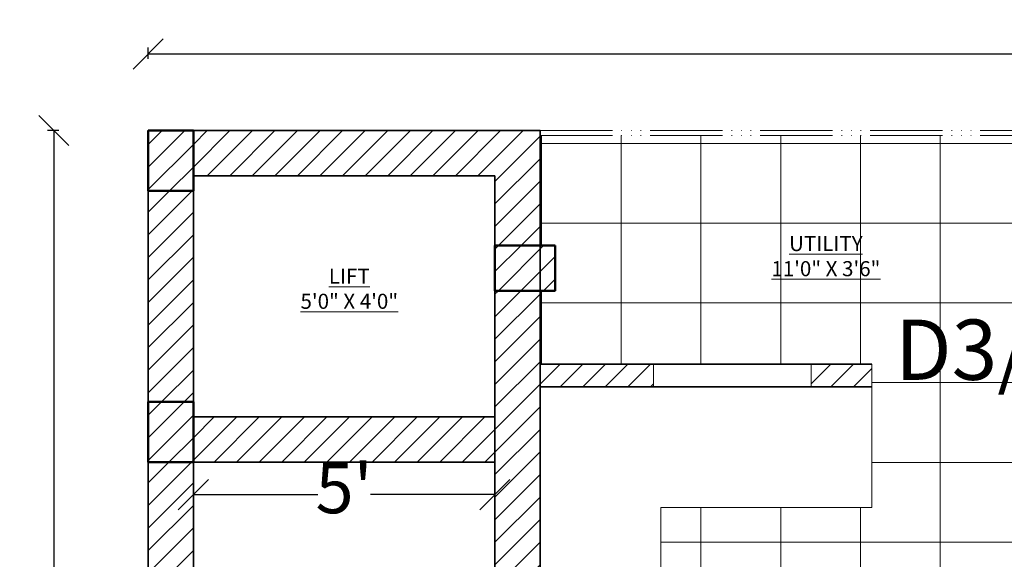
# Model space of a CAD drawing. Units: inches. Extents: x 2036 to 2670, y 319 to 920.
# Tile 4 of 15: x 2055 to 2251, y 790 to 898. Entities that reach past the tile are written whole.
import ezdxf

# ---------------------------------------------------------------- set-up
doc = ezdxf.new("R2010")
doc.units = ezdxf.units.IN
doc.linetypes.add('ACAD_ISO06W100', pattern=[36, 24, -3, 0, -3, 0, -3, 0, -3])
for name, color, linetype, lineweight in [('A-ANNO-DIMS', 2, 'Continuous', 18), ('A-ANNO-TEXT', 7, 'Continuous', 18), ('A-AREA-IDEN', 7, 'Continuous', 18), ('A-CASE', 7, 'Continuous', 18), ('A-COLS', 7, 'Continuous', 50), ('A-FLOR-EDGE', 5, 'ACAD_ISO06W100', 13), ('A-FLOR-PATT', 8, 'Continuous', 9), ('A-GLAZ', 4, 'Continuous', 18), ('A-WALL', 7, 'Continuous', 35)]:
    doc.layers.add(name, color=color, linetype=linetype, lineweight=lineweight)
doc.layers.add('A-COLS-PATT', color=240, linetype='Continuous', lineweight=13, true_color=0xed1f24)
doc.layers.add('A-WALL-PATT', color=52, linetype='Continuous', lineweight=13, true_color=0xc8c92d)
doc.styles.get("Standard").update_dxf_attribs({"font": 'arial.ttf'})
doc.dimstyles.new('ISO-25', dxfattribs={"dimtxt": 10, "dimasz": 6, "dimexe": 1.25, "dimexo": 0.625, "dimtad": 0, "dimdec": 1, "dimlunit": 3, "dimtxsty": 'Standard', "dimblk": 'OBLIQUE', "dimcen": 2.5, "dimclrd": 94, "dimclre": 94, "dimclrt": 1, "dimadec": 0, "dimazin": 0, "dimtfac": 1, "dimtdec": 1, "dimtmove": 0, "dimatfit": 3, "dimfxl": 1, "dimfxlon": 1, "dimarcsym": 0})

# ---------------------------------------------------------------- blocks, each defined once
blk = doc.blocks.new('_Oblique')
at = {"color": 0, "linetype": 'ByBlock', "lineweight": -2}
blk.add_line((-0.5, -0.5), (0.5, 0.5), dxfattribs=at)
blk = doc.blocks.new('*D10')
at = {"layer": 'A-ANNO-DIMS', "color": 0, "lineweight": -2, "transparency": 16777216}
for p, q in [((2080.74, 889.93), (2080.74, 892.18)), ((2612.74, 889.93), (2612.74, 892.18)), ((2080.74, 890.93), (2328.73, 890.93)), ((2612.74, 890.93), (2364.74, 890.93))]:
    blk.add_line(p, q, dxfattribs=at)
at = {"layer": 'Defpoints', "color": 0, "transparency": 16777216}
for p in [(2612.74, 890.93), (2080.74, 875.68), (2612.74, 875.68)]:
    blk.add_point(p, dxfattribs=at)
at = {"layer": 'A-ANNO-DIMS', "color": 0, "lineweight": -2, "transparency": 16777216, "xscale": 6, "yscale": 6, "zscale": 6, "rotation": 180}
blk.add_blockref('_Oblique', (2080.74, 890.93), dxfattribs=at)
at = {"layer": 'A-ANNO-DIMS', "color": 0, "lineweight": -2, "transparency": 16777216, "xscale": 6, "yscale": 6, "zscale": 6}
blk.add_blockref('_Oblique', (2612.74, 890.93), dxfattribs=at)
at = {"layer": 'A-ANNO-DIMS', "color": 0, "transparency": 16777216, "insert": (2346.74, 890.93), "char_height": 10, "attachment_point": 5}
blk.add_mtext('44\'-4"', dxfattribs=at)
blk = doc.blocks.new('*D13')
at = {"layer": 'A-ANNO-DIMS', "color": 0, "lineweight": -2, "transparency": 16777216}
for p, q in [((2062.98, 875.68), (2060.73, 875.68)), ((2061.98, 875.68), (2061.98, 687.98)), ((2061.98, 464.68), (2061.98, 652.39)), ((2062.98, 464.68), (2060.73, 464.68))]:
    blk.add_line(p, q, dxfattribs=at)
at = {"layer": 'Defpoints', "color": 0, "transparency": 16777216}
for p in [(2080.74, 875.68), (2061.98, 464.68), (2080.74, 464.68)]:
    blk.add_point(p, dxfattribs=at)
at = {"layer": 'A-ANNO-DIMS', "color": 0, "lineweight": -2, "transparency": 16777216, "xscale": 6, "yscale": 6, "zscale": 6}
for p, rotation in [((2061.98, 875.68), 90), ((2061.98, 464.68), 270)]:
    blk.add_blockref('_Oblique', p, dxfattribs=dict(at, rotation=rotation))
at = {"layer": 'A-ANNO-DIMS', "color": 0, "transparency": 16777216, "insert": (2061.98, 670.18), "char_height": 10, "attachment_point": 5, "rotation": 90}
blk.add_mtext('34\'-3"', dxfattribs=at)
blk = doc.blocks.new('*D14')
at = {"layer": 'A-ANNO-DIMS', "color": 0, "lineweight": -2, "transparency": 16777216}
for p, q in [((2089.74, 804.21), (2089.74, 801.96)), ((2149.74, 804.21), (2149.74, 801.96)), ((2089.74, 803.21), (2114.51, 803.21)), ((2149.74, 803.21), (2124.96, 803.21))]:
    blk.add_line(p, q, dxfattribs=at)
at = {"layer": 'Defpoints', "color": 0, "transparency": 16777216}
for p in [(2089.74, 809.68), (2149.74, 809.68), (2149.74, 803.21)]:
    blk.add_point(p, dxfattribs=at)
at = {"layer": 'A-ANNO-DIMS', "color": 0, "lineweight": -2, "transparency": 16777216, "xscale": 6, "yscale": 6, "zscale": 6, "rotation": 180}
blk.add_blockref('_Oblique', (2089.74, 803.21), dxfattribs=at)
at = {"layer": 'A-ANNO-DIMS', "color": 0, "lineweight": -2, "transparency": 16777216, "xscale": 6, "yscale": 6, "zscale": 6}
blk.add_blockref('_Oblique', (2149.74, 803.21), dxfattribs=at)
at = {"layer": 'A-ANNO-DIMS', "color": 0, "transparency": 16777216, "insert": (2119.74, 803.21), "char_height": 10, "attachment_point": 5}
blk.add_mtext("5'", dxfattribs=at)
blk = doc.blocks.new('COL-9x12')
blk.add_lwpolyline([(9, 0), (0, 0), (0, 12), (9, 12)], close=True)
blk = doc.blocks.new('*D58')
at = {"layer": 'A-ANNO-DIMS', "color": 94, "lineweight": -2, "transparency": 16777216}
for p, q in [((2224.74, 436.33), (2224.74, 434.08)), ((2224.74, 435.33), (2270.11, 435.33)), ((2270.11, 436.33), (2270.11, 434.08)), ((2270.11, 435.33), (2276.11, 435.33))]:
    blk.add_line(p, q, dxfattribs=at)
at = {"layer": 'Defpoints', "color": 0, "transparency": 16777216}
for p in [(2224.74, 824.68), (2270.11, 824.68), (2270.11, 435.33)]:
    blk.add_point(p, dxfattribs=at)
at = {"layer": 'A-ANNO-DIMS', "color": 94, "lineweight": -2, "transparency": 16777216, "xscale": 6, "yscale": 6, "zscale": 6, "rotation": 180}
blk.add_blockref('_Oblique', (2224.74, 435.33), dxfattribs=at)
at = {"layer": 'A-ANNO-DIMS', "color": 94, "lineweight": -2, "transparency": 16777216, "xscale": 6, "yscale": 6, "zscale": 6}
blk.add_blockref('_Oblique', (2270.11, 435.33), dxfattribs=at)
at = {"layer": 'A-ANNO-DIMS', "color": 1, "transparency": 16777216, "insert": (2301.68, 435.33), "char_height": 10, "attachment_point": 5}
blk.add_mtext('3\'-9 1/2"', dxfattribs=at)

msp = doc.modelspace()

# ---------------------------------------------------------------- hatches: boundary and pattern name
at = {"layer": 'A-COLS-PATT'}
h = msp.add_hatch(dxfattribs=at)
h.set_pattern_fill('ANSI31', color=256)
h.paths.add_polyline_path([(2089.74, 875.68), (2080.74, 875.68), (2080.74, 863.68), (2089.74, 863.68)])
h.paths.add_polyline_path([(2089.74, 821.68), (2080.74, 821.68), (2080.74, 809.68), (2089.74, 809.68)])
h.paths.add_polyline_path([(2089.74, 624.2), (2080.74, 624.2), (2080.74, 612.2), (2089.74, 612.2)])
h.paths.add_polyline_path([(2158.74, 506.68), (2149.74, 506.68), (2149.74, 494.68), (2158.74, 494.68)])
h.paths.add_polyline_path([(2158.74, 617.33), (2149.74, 617.33), (2149.74, 605.33), (2158.74, 605.33)])
h.paths.add_polyline_path([(2158.74, 736.18), (2149.74, 736.18), (2149.74, 724.18), (2158.74, 724.18)])
h.paths.add_polyline_path([(2158.74, 852.81), (2149.74, 852.81), (2149.74, 843.81), (2158.74, 843.81)])
h.paths.add_polyline_path([(2161.74, 852.81), (2158.74, 852.81), (2158.74, 843.81), (2161.74, 843.81)])
h.paths.add_polyline_path([(2295.21, 857.66), (2290.74, 857.66), (2290.74, 848.68), (2295.21, 848.68)])
h.paths.add_polyline_path([(2290.74, 857.66), (2283.21, 857.66), (2283.21, 848.66), (2290.74, 848.66)])
h.paths.add_polyline_path([(2443.62, 857.68), (2431.62, 857.68), (2431.62, 848.68), (2443.62, 848.68)])
h.paths.add_polyline_path([(2561.81, 857.68), (2549.81, 857.68), (2549.81, 848.68), (2561.81, 848.68)])
h.paths.add_polyline_path([(2295.24, 737.65), (2290.74, 737.65), (2290.74, 728.68), (2295.24, 728.68)])
h.paths.add_polyline_path([(2309.27, 612.12), (2297.27, 612.12), (2297.27, 603.12), (2309.27, 603.12)])
h.paths.add_polyline_path([(2282.24, 503.68), (2270.24, 503.68), (2270.24, 494.68), (2282.24, 494.68)])
h.paths.add_polyline_path([(2431.74, 746.09), (2427.24, 746.09), (2427.24, 737.09), (2431.74, 737.09)])
h.paths.add_polyline_path([(2439.24, 746.09), (2431.74, 746.09), (2431.74, 737.09), (2439.24, 737.09)])
h.paths.add_polyline_path([(2596.59, 736.59), (2584.59, 736.59), (2584.59, 727.59), (2596.59, 727.59)])
h.paths.add_polyline_path([(2586.39, 623.71), (2574.39, 623.71), (2574.39, 619.18), (2586.39, 619.18)])
h.paths.add_polyline_path([(2586.39, 619.18), (2574.39, 619.18), (2574.39, 614.71), (2586.39, 614.71)])
h.paths.add_polyline_path([(2438.74, 623.68), (2431.24, 623.68), (2431.24, 619.18), (2438.74, 619.18)])
h.paths.add_polyline_path([(2438.74, 619.18), (2431.24, 619.18), (2431.24, 614.68), (2438.74, 614.68)])
h.paths.add_polyline_path([(2431.24, 623.68), (2426.74, 623.68), (2426.74, 614.68), (2431.24, 614.68), (2431.24, 619.18)])
h.paths.add_polyline_path([(2527.24, 503.68), (2515.24, 503.68), (2515.24, 494.68), (2527.24, 494.68)])
h.paths.add_polyline_path([(2590.31, 503.68), (2578.31, 503.68), (2578.31, 494.68), (2590.31, 494.68)])
at = {"layer": 'A-FLOR-PATT'}
h = msp.add_hatch(dxfattribs=at)
h.set_pattern_fill('ANSI31', color=256, scale=5, angle=135)
h.paths.add_polyline_path([(2290.74, 659.68), (2158.74, 659.68), (2158.74, 582.53), (2158.74, 545.51), (2158.74, 503.68), (2426.74, 503.68), (2426.74, 614.68), (2426.74, 623.68), (2426.74, 628.18), (2431.24, 628.18), (2431.24, 623.68), (2438.74, 623.68), (2438.74, 619.18), (2574.39, 619.18), (2574.39, 623.71), (2586.39, 623.71), (2586.39, 619.18), (2603.74, 619.18), (2603.74, 824.68), (2431.74, 824.68), (2431.74, 746.09), (2439.24, 746.09), (2439.24, 737.09), (2431.74, 737.09), (2431.74, 659.68), (2427.24, 659.68), (2427.24, 739.48), (2383.24, 739.48), (2383.24, 804.68), (2339.24, 804.68), (2339.24, 749.08), (2295.24, 749.08), (2295.24, 737.65), (2295.27, 737.65), (2295.27, 728.65), (2295.21, 728.65, -0.586418), (2272.74, 728.68), (2272.74, 824.68), (2270.11, 824.68), (2270.11, 829.18), (2290.74, 829.18), (2290.74, 848.66), (2283.21, 848.66), (2283.21, 857.66), (2289.74, 857.66), (2289.74, 874.68), (2158.74, 874.68), (2158.74, 852.81), (2161.74, 852.81), (2161.74, 843.81), (2158.74, 843.81), (2158.74, 829.18), (2224.74, 829.18), (2224.74, 800.68), (2182.74, 800.68), (2182.74, 733.41), (2158.74, 733.41), (2158.74, 728.68), (2235.24, 728.68), (2235.24, 714.81), (2230.74, 714.81), (2230.74, 724.18), (2158.74, 724.18), (2158.74, 664.18), (2230.74, 664.18), (2230.74, 678.81), (2235.24, 678.81), (2235.24, 664.18), (2290.74, 664.18)])
h.paths.add_polyline_path([(2309.27, 612.12), (2309.27, 603.12), (2297.27, 603.12), (2297.27, 612.12)], flags=16)
h.paths.add_polyline_path([(2280.12, 639.11), (2280.26, 638.18, -0.414214), (2279.26, 637.18), (2278.76, 637.18), (2279.26, 633.18), (2277.76, 633.18), (2277.26, 637.18), (2269.76, 637.18), (2262.26, 637.18), (2261.76, 633.18), (2260.26, 633.18), (2260.76, 637.18), (2260.26, 637.18, -0.414214), (2259.26, 638.18), (2259.41, 639.11, -0.541164), (2257.76, 641.18), (2260.76, 652.18), (2261.45, 652.18), (2261.53, 652.68), (2262.76, 652.68), (2262.25, 655.24, 0.001913), (2261.76, 655.18), (2259.76, 658.18, -0.15), (2279.76, 658.18), (2277.76, 655.18, 0.001913), (2277.27, 655.24), (2276.76, 652.68), (2278, 652.68), (2278.07, 652.18), (2278.76, 652.18), (2281.76, 641.18, -0.541163)], flags=16)
h.paths.add_polyline_path([(2245.98, 639.11), (2246.13, 638.18, -0.414214), (2245.13, 637.18), (2244.63, 637.18), (2245.13, 633.18), (2243.63, 633.18), (2243.13, 637.18), (2235.63, 637.18), (2228.13, 637.18), (2227.63, 633.18), (2226.13, 633.18), (2226.63, 637.18), (2226.13, 637.18, -0.414214), (2225.13, 638.18), (2225.27, 639.11, -0.541164), (2223.63, 641.18), (2226.63, 652.18), (2227.32, 652.18), (2227.39, 652.68), (2228.63, 652.68), (2228.12, 655.24, 0.001913), (2227.63, 655.18), (2225.63, 658.18, -0.15), (2245.63, 658.18), (2243.63, 655.18, 0.001913), (2243.14, 655.24), (2242.63, 652.68), (2243.86, 652.68), (2243.94, 652.18), (2244.63, 652.18), (2247.63, 641.18, -0.541163)], flags=16)
h.paths.add_polyline_path([(2351.59, 515.15, -0.151948), (2279.59, 515.15), (2279.59, 537.68), (2273.59, 537.68), (2273.59, 511.68, 0.190476), (2357.59, 511.68), (2357.59, 537.68), (2351.59, 537.68)])
h.paths.add_polyline_path([(2327.59, 536.13), (2327.59, 517.07), (2303.59, 517.07), (2303.59, 536.13)], flags=16)
h.paths.add_polyline_path([(2213.4, 639.11), (2213.55, 638.18, -0.414214), (2212.55, 637.18), (2212.05, 637.18), (2212.55, 633.18), (2211.05, 633.18), (2210.55, 637.18), (2203.05, 637.18), (2195.55, 637.18), (2195.05, 633.18), (2193.55, 633.18), (2194.05, 637.18), (2193.55, 637.18, -0.414214), (2192.55, 638.18), (2192.69, 639.11, -0.541164), (2191.05, 641.18), (2194.05, 652.18), (2194.73, 652.18), (2194.81, 652.68), (2196.05, 652.68), (2195.53, 655.24, 0.001913), (2195.05, 655.18), (2193.05, 658.18, -0.15), (2213.05, 658.18), (2211.05, 655.18, 0.001913), (2210.56, 655.24), (2210.05, 652.68), (2211.28, 652.68), (2211.36, 652.18), (2212.05, 652.18), (2215.05, 641.18, -0.541163)], flags=16)
h.paths.add_polyline_path([(2368.58, 538.02), (2370.52, 538.02), (2371.17, 532.84), (2380.89, 532.84), (2390.6, 532.84), (2391.25, 538.02), (2393.2, 538.02), (2392.55, 532.84), (2380.89, 532.84), (2368.58, 532.84, 0.414214), (2367.28, 531.54), (2367.47, 530.34, -0.483352), (2369.23, 527.65), (2371.82, 513.4), (2370.12, 513.4), (2370.22, 512.75), (2391.56, 512.75), (2391.66, 513.4), (2389.96, 513.4), (2392.55, 527.65, -1.387427), (2396.43, 527.65), (2392.55, 513.4), (2391.66, 513.4), (2391.56, 512.75), (2389.31, 512.75), (2390, 509.37, 0.003796), (2391.25, 509.51), (2393.84, 505.63, -0.15), (2367.93, 505.63), (2370.52, 509.51, 0.003901), (2371.81, 509.36), (2372.47, 512.75), (2370.22, 512.75), (2370.12, 513.4), (2369.23, 513.4), (2365.34, 527.65, -0.541163), (2367.47, 530.34), (2367.28, 531.54, -0.414214), (2368.58, 532.84), (2369.23, 532.84)])
h.paths.add_polyline_path([(2266.74, 538.02), (2266.09, 532.84), (2254.43, 532.84), (2242.12, 532.84, 0.414214), (2240.83, 531.54), (2241.01, 530.34, -0.483352), (2242.77, 527.65), (2245.36, 513.4), (2243.66, 513.4), (2243.76, 512.75), (2265.1, 512.75), (2265.2, 513.4), (2263.5, 513.4), (2266.09, 527.65, -1.387427), (2269.98, 527.65), (2266.09, 513.4), (2265.2, 513.4), (2265.1, 512.75), (2262.85, 512.75), (2263.54, 509.37, 0.003796), (2264.79, 509.51), (2267.39, 505.63, -0.15), (2241.47, 505.63), (2244.07, 509.51, 0.003901), (2245.36, 509.36), (2246.01, 512.75), (2243.76, 512.75), (2243.66, 513.4), (2242.77, 513.4), (2238.88, 527.65, -0.541163), (2241.01, 530.34), (2240.83, 531.54, -0.414214), (2242.12, 532.84), (2242.77, 532.84), (2242.12, 538.02), (2244.07, 538.02), (2244.71, 532.84), (2254.43, 532.84), (2264.15, 532.84), (2264.79, 538.02)])
h.paths.add_polyline_path([(2185.24, 620.36), (2185.24, 618.86), (2181.24, 618.36), (2181.24, 610.86), (2181.24, 603.36), (2185.24, 602.86), (2185.24, 601.36), (2181.24, 601.86), (2181.24, 601.36, -0.414214), (2180.24, 600.36), (2179.31, 600.5, -0.541164), (2177.24, 598.86), (2166.24, 601.86), (2166.24, 602.54), (2165.74, 602.62), (2165.74, 603.86), (2163.18, 603.34, 0.001913), (2163.24, 602.86), (2160.24, 600.86, -0.15), (2160.24, 620.86), (2163.24, 618.86, 0.001913), (2163.18, 618.37), (2165.74, 617.86), (2165.74, 619.09), (2166.24, 619.17), (2166.24, 619.86), (2177.24, 622.86, -0.541163), (2179.31, 621.21), (2180.24, 621.36, -0.414214), (2181.24, 620.36), (2181.24, 619.86)])
h.paths.add_polyline_path([(2470.92, 676.01), (2470.92, 806.13), (2568.52, 806.13), (2568.52, 676.01)], flags=16)
h.paths.add_polyline_path([(2177.74, 677.49), (2161.9, 677.49), (2161.9, 705.85), (2177.74, 705.85)], flags=16)
h.paths.add_polyline_path([(2176.74, 678.49), (2162.9, 678.49), (2162.9, 704.85), (2176.74, 704.85)], flags=0)
h.paths.add_polyline_path([(2175.01, 686.48), (2172.93, 686.48), (2172.93, 690.63), (2170.86, 690.63), (2170.86, 686.48), (2164.63, 686.48), (2164.63, 688.56), (2166.71, 688.56), (2168.78, 688.56), (2168.78, 690.63), (2164.63, 690.63), (2164.63, 696.85), (2166.71, 696.85), (2166.71, 692.71), (2168.78, 692.71), (2168.78, 696.85), (2175.01, 696.85), (2175.01, 694.78), (2170.86, 694.78), (2170.86, 692.71), (2175.01, 692.71)], flags=0)
h.paths.add_polyline_path([(2543.79, 782.71), (2483.94, 782.71), (2483.94, 804.18), (2517.77, 804.18), (2517.77, 782.71), (2521.67, 782.71), (2521.67, 804.18), (2555.5, 804.18), (2555.5, 779.45), (2547.05, 779.45), (2568.52, 757.98), (2543.79, 757.98)], flags=0)
h.paths.add_polyline_path([(2584.59, 727.59), (2584.59, 736.59), (2596.59, 736.59), (2596.59, 727.59)], flags=16)
h.paths.add_polyline_path([(2520.45, 647.03), (2553.79, 647.03), (2553.79, 658.23), (2520.45, 658.23)], flags=24)
h.paths.add_polyline_path([(2299.53, 573.74), (2331.71, 573.74), (2331.71, 584.94), (2299.53, 584.94)], flags=24)
h.paths.add_polyline_path([(2191.59, 685.19), (2212.12, 685.19), (2212.12, 696.38), (2191.59, 696.38)], flags=24)
h.paths.add_polyline_path([(2353.9, 649.86), (2379.08, 649.86), (2379.08, 661.06), (2353.9, 661.06)], flags=24)
h.paths.add_polyline_path([(2214.61, 763.31), (2237.46, 763.31), (2237.46, 779.56), (2214.61, 779.56)], flags=24)
h.paths.add_polyline_path([(2225.09, 819.31), (2269.29, 819.31), (2269.29, 844.04), (2225.09, 844.04)], flags=24)
h.paths.add_polyline_path([(2204.06, 845.04), (2226.92, 845.04), (2226.92, 856.24), (2204.06, 856.24)], flags=24)
h = msp.add_hatch(dxfattribs=at)
h.set_pattern_fill('ANSI31', color=256, scale=5, angle=45)
h.paths.add_polyline_path([(2290.74, 659.68), (2158.74, 659.68), (2158.74, 582.53), (2158.74, 545.51), (2158.74, 503.68), (2426.74, 503.68), (2426.74, 614.68), (2426.74, 623.68), (2426.74, 628.18), (2431.24, 628.18), (2431.24, 623.68), (2438.74, 623.68), (2438.74, 619.18), (2574.39, 619.18), (2574.39, 623.71), (2586.39, 623.71), (2586.39, 619.18), (2603.74, 619.18), (2603.74, 824.68), (2431.74, 824.68), (2431.74, 746.09), (2439.24, 746.09), (2439.24, 737.09), (2431.74, 737.09), (2431.74, 659.68), (2427.24, 659.68), (2427.24, 739.48), (2383.24, 739.48), (2383.24, 804.68), (2339.24, 804.68), (2339.24, 749.08), (2295.24, 749.08), (2295.24, 737.65), (2295.27, 737.65), (2295.27, 728.65), (2295.21, 728.65, -0.586418), (2272.74, 728.68), (2272.74, 824.68), (2270.11, 824.68), (2270.11, 829.18), (2290.74, 829.18), (2290.74, 848.66), (2283.21, 848.66), (2283.21, 857.66), (2289.74, 857.66), (2289.74, 874.68), (2158.74, 874.68), (2158.74, 852.81), (2161.74, 852.81), (2161.74, 843.81), (2158.74, 843.81), (2158.74, 829.18), (2224.74, 829.18), (2224.74, 800.68), (2182.74, 800.68), (2182.74, 733.41), (2158.74, 733.41), (2158.74, 728.68), (2235.24, 728.68), (2235.24, 714.81), (2230.74, 714.81), (2230.74, 724.18), (2158.74, 724.18), (2158.74, 664.18), (2230.74, 664.18), (2230.74, 678.81), (2235.24, 678.81), (2235.24, 664.18), (2290.74, 664.18)])
h.paths.add_polyline_path([(2309.27, 612.12), (2309.27, 603.12), (2297.27, 603.12), (2297.27, 612.12)], flags=16)
h.paths.add_polyline_path([(2280.12, 639.11), (2280.26, 638.18, -0.414214), (2279.26, 637.18), (2278.76, 637.18), (2279.26, 633.18), (2277.76, 633.18), (2277.26, 637.18), (2269.76, 637.18), (2262.26, 637.18), (2261.76, 633.18), (2260.26, 633.18), (2260.76, 637.18), (2260.26, 637.18, -0.414214), (2259.26, 638.18), (2259.41, 639.11, -0.541164), (2257.76, 641.18), (2260.76, 652.18), (2261.45, 652.18), (2261.53, 652.68), (2262.76, 652.68), (2262.25, 655.24, 0.001913), (2261.76, 655.18), (2259.76, 658.18, -0.15), (2279.76, 658.18), (2277.76, 655.18, 0.001913), (2277.27, 655.24), (2276.76, 652.68), (2278, 652.68), (2278.07, 652.18), (2278.76, 652.18), (2281.76, 641.18, -0.541163)], flags=16)
h.paths.add_polyline_path([(2245.98, 639.11), (2246.13, 638.18, -0.414214), (2245.13, 637.18), (2244.63, 637.18), (2245.13, 633.18), (2243.63, 633.18), (2243.13, 637.18), (2235.63, 637.18), (2228.13, 637.18), (2227.63, 633.18), (2226.13, 633.18), (2226.63, 637.18), (2226.13, 637.18, -0.414214), (2225.13, 638.18), (2225.27, 639.11, -0.541164), (2223.63, 641.18), (2226.63, 652.18), (2227.32, 652.18), (2227.39, 652.68), (2228.63, 652.68), (2228.12, 655.24, 0.001913), (2227.63, 655.18), (2225.63, 658.18, -0.15), (2245.63, 658.18), (2243.63, 655.18, 0.001913), (2243.14, 655.24), (2242.63, 652.68), (2243.86, 652.68), (2243.94, 652.18), (2244.63, 652.18), (2247.63, 641.18, -0.541163)], flags=16)
h.paths.add_polyline_path([(2351.59, 537.68), (2351.59, 515.15, -0.151948), (2279.59, 515.15), (2279.59, 537.68), (2273.59, 537.68), (2273.59, 511.68, 0.190476), (2357.59, 511.68), (2357.59, 537.68)])
h.paths.add_polyline_path([(2368.58, 538.02), (2370.52, 538.02), (2371.17, 532.84), (2380.89, 532.84), (2390.6, 532.84), (2391.25, 538.02), (2393.2, 538.02), (2392.55, 532.84), (2380.89, 532.84), (2368.58, 532.84, 0.414214), (2367.28, 531.54), (2367.47, 530.34, -0.483352), (2369.23, 527.65), (2371.82, 513.4), (2370.12, 513.4), (2370.22, 512.75), (2391.56, 512.75), (2391.66, 513.4), (2389.96, 513.4), (2392.55, 527.65, -1.387427), (2396.43, 527.65), (2392.55, 513.4), (2391.66, 513.4), (2391.56, 512.75), (2389.31, 512.75), (2390, 509.37, 0.003796), (2391.25, 509.51), (2393.84, 505.63, -0.15), (2367.93, 505.63), (2370.52, 509.51, 0.003901), (2371.81, 509.36), (2372.47, 512.75), (2370.22, 512.75), (2370.12, 513.4), (2369.23, 513.4), (2365.34, 527.65, -0.541163), (2367.47, 530.34), (2367.28, 531.54, -0.414214), (2368.58, 532.84), (2369.23, 532.84)])
h.paths.add_polyline_path([(2327.59, 536.13), (2327.59, 517.07), (2303.59, 517.07), (2303.59, 536.13)], flags=16)
h.paths.add_polyline_path([(2470.92, 676.01), (2470.92, 806.13), (2568.52, 806.13), (2568.52, 676.01)], flags=16)
h.paths.add_polyline_path([(2266.74, 538.02), (2266.09, 532.84), (2254.43, 532.84), (2242.12, 532.84, 0.414214), (2240.83, 531.54), (2241.01, 530.34, -0.483352), (2242.77, 527.65), (2245.36, 513.4), (2243.66, 513.4), (2243.76, 512.75), (2265.1, 512.75), (2265.2, 513.4), (2263.5, 513.4), (2266.09, 527.65, -1.387427), (2269.98, 527.65), (2266.09, 513.4), (2265.2, 513.4), (2265.1, 512.75), (2262.85, 512.75), (2263.54, 509.37, 0.003796), (2264.79, 509.51), (2267.39, 505.63, -0.15), (2241.47, 505.63), (2244.07, 509.51, 0.003901), (2245.36, 509.36), (2246.01, 512.75), (2243.76, 512.75), (2243.66, 513.4), (2242.77, 513.4), (2238.88, 527.65, -0.541163), (2241.01, 530.34), (2240.83, 531.54, -0.414214), (2242.12, 532.84), (2242.77, 532.84), (2242.12, 538.02), (2244.07, 538.02), (2244.71, 532.84), (2254.43, 532.84), (2264.15, 532.84), (2264.79, 538.02)])
h.paths.add_polyline_path([(2213.4, 639.11), (2213.55, 638.18, -0.414214), (2212.55, 637.18), (2212.05, 637.18), (2212.55, 633.18), (2211.05, 633.18), (2210.55, 637.18), (2203.05, 637.18), (2195.55, 637.18), (2195.05, 633.18), (2193.55, 633.18), (2194.05, 637.18), (2193.55, 637.18, -0.414214), (2192.55, 638.18), (2192.69, 639.11, -0.541164), (2191.05, 641.18), (2194.05, 652.18), (2194.73, 652.18), (2194.81, 652.68), (2196.05, 652.68), (2195.53, 655.24, 0.001913), (2195.05, 655.18), (2193.05, 658.18, -0.15), (2213.05, 658.18), (2211.05, 655.18, 0.001913), (2210.56, 655.24), (2210.05, 652.68), (2211.28, 652.68), (2211.36, 652.18), (2212.05, 652.18), (2215.05, 641.18, -0.541163)], flags=16)
h.paths.add_polyline_path([(2185.24, 620.36), (2185.24, 618.86), (2181.24, 618.36), (2181.24, 610.86), (2181.24, 603.36), (2185.24, 602.86), (2185.24, 601.36), (2181.24, 601.86), (2181.24, 601.36, -0.414214), (2180.24, 600.36), (2179.31, 600.5, -0.541164), (2177.24, 598.86), (2166.24, 601.86), (2166.24, 602.54), (2165.74, 602.62), (2165.74, 603.86), (2163.18, 603.34, 0.001913), (2163.24, 602.86), (2160.24, 600.86, -0.15), (2160.24, 620.86), (2163.24, 618.86, 0.001913), (2163.18, 618.37), (2165.74, 617.86), (2165.74, 619.09), (2166.24, 619.17), (2166.24, 619.86), (2177.24, 622.86, -0.541163), (2179.31, 621.21), (2180.24, 621.36, -0.414214), (2181.24, 620.36), (2181.24, 619.86)])
h.paths.add_polyline_path([(2177.74, 677.49), (2161.9, 677.49), (2161.9, 705.85), (2177.74, 705.85)], flags=16)
h.paths.add_polyline_path([(2176.74, 678.49), (2162.9, 678.49), (2162.9, 704.85), (2176.74, 704.85)], flags=0)
h.paths.add_polyline_path([(2175.01, 686.48), (2172.93, 686.48), (2172.93, 690.63), (2170.86, 690.63), (2170.86, 686.48), (2164.63, 686.48), (2164.63, 688.56), (2166.71, 688.56), (2168.78, 688.56), (2168.78, 690.63), (2164.63, 690.63), (2164.63, 696.85), (2166.71, 696.85), (2166.71, 692.71), (2168.78, 692.71), (2168.78, 696.85), (2175.01, 696.85), (2175.01, 694.78), (2170.86, 694.78), (2170.86, 692.71), (2175.01, 692.71)], flags=0)
h.paths.add_polyline_path([(2543.79, 782.71), (2483.94, 782.71), (2483.94, 804.18), (2517.77, 804.18), (2517.77, 782.71), (2521.67, 782.71), (2521.67, 804.18), (2555.5, 804.18), (2555.5, 779.45), (2547.05, 779.45), (2568.52, 757.98), (2543.79, 757.98)], flags=0)
h.paths.add_polyline_path([(2584.59, 727.59), (2584.59, 736.59), (2596.59, 736.59), (2596.59, 727.59)], flags=16)
h.paths.add_polyline_path([(2520.45, 647.03), (2553.79, 647.03), (2553.79, 658.23), (2520.45, 658.23)], flags=24)
h.paths.add_polyline_path([(2299.53, 573.74), (2331.71, 573.74), (2331.71, 584.94), (2299.53, 584.94)], flags=24)
h.paths.add_polyline_path([(2191.59, 685.19), (2212.12, 685.19), (2212.12, 696.38), (2191.59, 696.38)], flags=24)
h.paths.add_polyline_path([(2353.9, 649.86), (2379.08, 649.86), (2379.08, 661.06), (2353.9, 661.06)], flags=24)
h.paths.add_polyline_path([(2214.61, 763.31), (2237.46, 763.31), (2237.46, 779.56), (2214.61, 779.56)], flags=24)
h.paths.add_polyline_path([(2225.09, 819.31), (2269.29, 819.31), (2269.29, 844.04), (2225.09, 844.04)], flags=24)
h.paths.add_polyline_path([(2204.06, 845.04), (2226.92, 845.04), (2226.92, 856.24), (2204.06, 856.24)], flags=24)
at = {"layer": 'A-WALL-PATT'}
h = msp.add_hatch(dxfattribs=at)
h.set_pattern_fill('ANSI31', color=256)
h.paths.add_polyline_path([(2089.74, 863.68), (2080.74, 863.68), (2080.74, 821.68), (2089.74, 821.68)])
h.paths.add_polyline_path([(2089.74, 809.68), (2080.74, 809.68), (2080.74, 624.2), (2089.74, 624.2), (2089.74, 707.68), (2089.74, 767.68)])
h.paths.add_polyline_path([(2149.74, 818.68), (2089.74, 818.68), (2089.74, 809.68), (2149.74, 809.68)])
h.paths.add_polyline_path([(2158.74, 875.68), (2089.74, 875.68), (2089.74, 866.68), (2149.74, 866.68), (2149.74, 852.81), (2158.74, 852.81)])
h.paths.add_polyline_path([(2158.74, 843.81), (2149.74, 843.81), (2149.74, 736.18), (2158.74, 736.18), (2158.74, 824.68)])
h.paths.add_polyline_path([(2181.31, 829.18), (2158.74, 829.18), (2158.74, 824.68), (2181.31, 824.68)])
h.paths.add_polyline_path([(2224.74, 829.18), (2212.72, 829.18), (2212.72, 824.68), (2224.74, 824.68)])
h.paths.add_polyline_path([(2177.02, 503.68), (2158.74, 503.68), (2158.74, 494.68), (2177.02, 494.68)])
h.paths.add_polyline_path([(2158.74, 664.18), (2158.74, 680.02), (2149.74, 680.02), (2149.74, 617.33), (2158.74, 617.33)])
h.paths.add_polyline_path([(2158.74, 724.18), (2149.74, 724.18), (2149.74, 704.02), (2158.74, 704.02)])
h.paths.add_polyline_path([(2235.24, 728.68), (2158.74, 728.68), (2158.74, 724.18), (2230.74, 724.18), (2230.74, 714.81), (2235.24, 714.81)])
h.paths.add_polyline_path([(2290.74, 664.18), (2235.24, 664.18), (2235.24, 678.81), (2230.74, 678.81), (2230.74, 664.18), (2158.74, 664.18), (2158.74, 659.68), (2290.74, 659.68)])
h.paths.add_polyline_path([(2270.24, 503.68), (2227.17, 503.68), (2227.17, 494.68), (2270.24, 494.68)])
h.paths.add_polyline_path([(2515.24, 503.68), (2380.89, 503.68), (2380.89, 494.68), (2515.24, 494.68)])
h.paths.add_polyline_path([(2292.21, 503.68), (2282.24, 503.68), (2282.24, 494.68), (2292.21, 494.68)])
h.paths.add_polyline_path([(2578.31, 503.68), (2527.24, 503.68), (2527.24, 494.68), (2578.31, 494.68)])
h.paths.add_polyline_path([(2603.74, 503.68), (2590.31, 503.68), (2590.31, 494.68), (2603.74, 494.68)])
h.paths.add_polyline_path([(2612.74, 503.68), (2603.74, 503.68), (2603.74, 494.68), (2612.74, 494.68)])
h.paths.add_polyline_path([(2549.81, 857.68), (2443.62, 857.68), (2443.62, 848.68), (2549.81, 848.68)])
h.paths.add_polyline_path([(2295.24, 848.66), (2290.74, 848.66), (2290.74, 829.18), (2270.11, 829.18), (2270.11, 824.68), (2290.74, 824.68), (2290.74, 737.65), (2295.24, 737.65)])
h.paths.add_polyline_path([(2431.74, 737.09), (2427.24, 737.09), (2427.24, 659.68), (2431.74, 659.68)])
h.paths.add_polyline_path([(2431.74, 848.68), (2427.24, 848.68), (2427.24, 746.09), (2431.74, 746.09)])
h.paths.add_polyline_path([(2574.39, 619.18), (2495.46, 619.18), (2495.46, 614.68), (2574.39, 614.68)])
h.paths.add_polyline_path([(2461.84, 619.18), (2438.74, 619.18), (2438.74, 614.68), (2461.84, 614.68)])
h.paths.add_polyline_path([(2603.74, 619.18), (2586.39, 619.18), (2586.39, 614.68), (2603.74, 614.68)], flags=17)

# ---------------------------------------------------------------- linework, layer by layer
at = {"layer": 'A-CASE'}
for p, q in [((2224.74, 800.68), (2224.74, 829.18)), ((2182.74, 800.68), (2182.74, 733.41)), ((2182.74, 800.68), (2224.74, 800.68)), ((2182.74, 800.68), (2224.74, 800.68))]:
    msp.add_line(p, q, dxfattribs=at)
at = {"layer": 'A-COLS'}
for points in [[(2089.74, 863.68), (2080.74, 863.68), (2080.74, 875.68), (2089.74, 875.68)], [(2089.74, 809.68), (2080.74, 809.68), (2080.74, 821.68), (2089.74, 821.68)]]:
    msp.add_lwpolyline(points, close=True, dxfattribs=at)
at = {"layer": 'A-FLOR-EDGE', "ltscale": 0.6}
for p, q in [((2158.74, 875.68), (2290.74, 875.68)), ((2158.74, 874.68), (2289.74, 874.68))]:
    msp.add_line(p, q, dxfattribs=at)
at = {"layer": 'A-GLAZ'}
for p, q in [((2181.31, 829.18), (2181.31, 824.68)), ((2212.72, 829.18), (2212.72, 824.68))]:
    msp.add_line(p, q, dxfattribs=at)
at = {"layer": 'A-WALL'}
for p, q in [((2158.74, 875.68), (2080.74, 875.68)), ((2080.74, 875.68), (2080.74, 599.68)), ((2158.74, 875.68), (2158.74, 824.68)), ((2089.74, 866.68), (2089.74, 767.68)), ((2149.74, 866.68), (2089.74, 866.68)), ((2149.74, 866.68), (2149.74, 582.53)), ((2158.74, 829.18), (2224.74, 829.18)), ((2158.74, 824.68), (2224.74, 824.68)), ((2158.74, 824.68), (2158.74, 728.68)), ((2149.74, 818.68), (2089.74, 818.68)), ((2149.74, 809.68), (2089.74, 809.68))]:
    msp.add_line(p, q, dxfattribs=at)

# ---------------------------------------------------------------- block references
at = {"layer": 'A-COLS', "rotation": 89.99999999999625}
msp.add_blockref('COL-9x12', (2161.74, 843.81), dxfattribs=at)

# ---------------------------------------------------------------- texts
at = {"layer": 'A-ANNO-TEXT', "insert": (2229.39, 838.06), "char_height": 12, "attachment_point": 1}
msp.add_mtext_dynamic_manual_height_columns('D3/C', width=19.553, gutter_width=12.5, heights=[0], dxfattribs=at)
at = {"layer": 'A-AREA-IDEN', "char_height": 3, "attachment_point": 1}
for s, insert in [('\\pxqc;{\\LUTILITY\\P11\'0" X 3\'6"}', (2203.58, 854.69)), ('\\pxqc;{\\LLIFT\\P5\'0" X 4\'0"}', (2108.73, 848.2))]:
    msp.add_mtext_dynamic_manual_height_columns(s, width=24.0713, gutter_width=12.5, heights=[0], dxfattribs=dict(at, insert=insert))

# ---------------------------------------------------------------- dimensions: what is measured, and where the dimension line sits
at = {"layer": 'A-ANNO-DIMS'}
for base, p1, p2, override, picture, middle in [((2612.74, 890.93), (2080.74, 875.68), (2612.74, 875.68), {"dimclrd": 0, "dimclre": 0, "dimclrt": 0}, '*D10', (2346.74, 890.93)), ((2270.11, 435.33), (2224.74, 824.68), (2270.11, 824.68), {"dimdec": 1, "dimlfac": 1, "dimrnd": 0, "dimzin": 1, "dimdsep": 46, "dimlunit": 4, "dimfrac": 2}, '*D58', (2301.68, 435.33)), ((2149.74, 803.21), (2089.74, 809.68), (2149.74, 809.68), {"dimclrd": 0, "dimclre": 0, "dimclrt": 0}, '*D14', (2119.74, 803.21))]:
    dim = msp.add_linear_dim(base=base, p1=p1, p2=p2, dimstyle='ISO-25', override=override, dxfattribs=at)
    dim.commit()
    dim.dimension.update_dxf_attribs({"geometry": picture, "text_midpoint": middle})
dim = msp.add_linear_dim(base=(2061.98, 464.68), p1=(2080.74, 875.68), p2=(2080.74, 464.68), angle=90, dimstyle='ISO-25', override={"dimclrd": 0, "dimclre": 0, "dimclrt": 0}, dxfattribs=at)
dim.commit()
dim.dimension.update_dxf_attribs({"geometry": '*D13', "text_midpoint": (2061.98, 670.18)})

doc.saveas('drawing.dxf')
